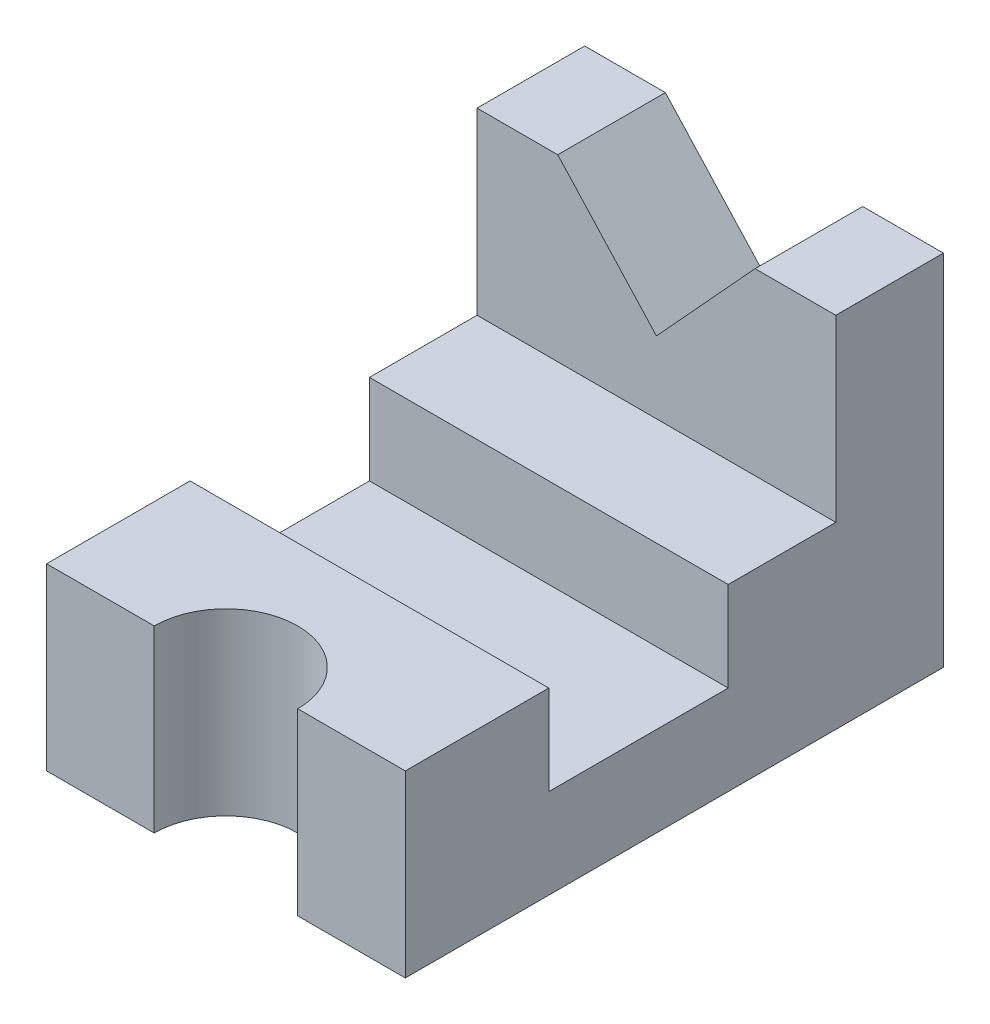
ISO-10303-21;
HEADER;
FILE_DESCRIPTION(('STEP AP214'),'2;1');
FILE_NAME('part.step','',(''),(''),'','','');
FILE_SCHEMA(('AUTOMOTIVE_DESIGN { 1 0 10303 214 1 1 1 1 }'));
ENDSEC;
DATA;
#1=APPLICATION_CONTEXT('core data for automotive mechanical design processes');
#2=APPLICATION_PROTOCOL_DEFINITION('international standard','automotive_design',2000,#1);
#3=PRODUCT_CONTEXT('',#1,'mechanical');
#4=PRODUCT('Part','Part','',(#3));
#5=PRODUCT_RELATED_PRODUCT_CATEGORY('part','',(#4));
#6=PRODUCT_DEFINITION_FORMATION('','',#4);
#7=PRODUCT_DEFINITION_CONTEXT('part definition',#1,'design');
#8=PRODUCT_DEFINITION('design','',#6,#7);
#9=PRODUCT_DEFINITION_SHAPE('','',#8);
#10=(LENGTH_UNIT() NAMED_UNIT(*) SI_UNIT(.MILLI.,.METRE.));
#11=(NAMED_UNIT(*) PLANE_ANGLE_UNIT() SI_UNIT($,.RADIAN.));
#12=(NAMED_UNIT(*) SI_UNIT($,.STERADIAN.) SOLID_ANGLE_UNIT());
#13=UNCERTAINTY_MEASURE_WITH_UNIT(LENGTH_MEASURE(1.E-05),#10,'distance_accuracy_value','');
#14=(GEOMETRIC_REPRESENTATION_CONTEXT(3) GLOBAL_UNCERTAINTY_ASSIGNED_CONTEXT((#13)) GLOBAL_UNIT_ASSIGNED_CONTEXT((#10,
#11,#12)) REPRESENTATION_CONTEXT('',''));
#15=CARTESIAN_POINT('',(0.,0.,0.));
#16=DIRECTION('',(0.,0.,1.));
#17=DIRECTION('',(1.,0.,0.));
#18=AXIS2_PLACEMENT_3D('',#15,#16,#17);
#19=CARTESIAN_POINT('',(60.,40.,12.));
#20=DIRECTION('',(0.,1.,0.));
#21=DIRECTION('',(0.,0.,1.));
#22=AXIS2_PLACEMENT_3D('',#19,#20,#21);
#23=PLANE('',#22);
#24=DIRECTION('',(0.,0.,1.));
#25=VECTOR('',#24,1.);
#26=CARTESIAN_POINT('',(51.,40.,-48.));
#27=LINE('',#26,#25);
#28=CARTESIAN_POINT('',(51.,40.,0.));
#29=VERTEX_POINT('',#28);
#30=CARTESIAN_POINT('',(51.,40.,12.));
#31=VERTEX_POINT('',#30);
#32=EDGE_CURVE('E157',#29,#31,#27,.T.);
#33=ORIENTED_EDGE('',*,*,#32,.T.);
#34=DIRECTION('',(1.,0.,0.));
#35=VECTOR('',#34,1.);
#36=CARTESIAN_POINT('',(60.,40.,12.));
#37=LINE('',#36,#35);
#38=CARTESIAN_POINT('',(60.,40.,12.));
#39=VERTEX_POINT('',#38);
#40=EDGE_CURVE('E168',#31,#39,#37,.T.);
#41=ORIENTED_EDGE('',*,*,#40,.T.);
#42=DIRECTION('',(0.,0.,-1.));
#43=VECTOR('',#42,1.);
#44=CARTESIAN_POINT('',(60.,40.,12.));
#45=LINE('',#44,#43);
#46=CARTESIAN_POINT('',(60.,40.,0.));
#47=VERTEX_POINT('',#46);
#48=EDGE_CURVE('E229',#39,#47,#45,.T.);
#49=ORIENTED_EDGE('',*,*,#48,.T.);
#50=DIRECTION('',(1.,0.,0.));
#51=VECTOR('',#50,1.);
#52=CARTESIAN_POINT('',(60.,40.,0.));
#53=LINE('',#52,#51);
#54=EDGE_CURVE('E221',#29,#47,#53,.T.);
#55=ORIENTED_EDGE('',*,*,#54,.F.);
#56=EDGE_LOOP('',(#33,#41,#49,#55));
#57=FACE_BOUND('',#56,.T.);
#58=ADVANCED_FACE('F44',(#57),#23,.T.);
#59=CARTESIAN_POINT('',(0.,20.,60.));
#60=DIRECTION('',(0.,-1.,0.));
#61=DIRECTION('',(0.,0.,-1.));
#62=AXIS2_PLACEMENT_3D('',#59,#60,#61);
#63=PLANE('',#62);
#64=DIRECTION('',(0.,0.,-1.));
#65=VECTOR('',#64,1.);
#66=CARTESIAN_POINT('',(60.,20.,60.));
#67=LINE('',#66,#65);
#68=CARTESIAN_POINT('',(60.,20.,60.));
#69=VERTEX_POINT('',#68);
#70=CARTESIAN_POINT('',(60.,20.,44.));
#71=VERTEX_POINT('',#70);
#72=EDGE_CURVE('E247',#69,#71,#67,.T.);
#73=ORIENTED_EDGE('',*,*,#72,.T.);
#74=DIRECTION('',(1.,0.,0.));
#75=VECTOR('',#74,1.);
#76=CARTESIAN_POINT('',(0.,20.,44.));
#77=LINE('',#76,#75);
#78=CARTESIAN_POINT('',(20.,20.,44.));
#79=VERTEX_POINT('',#78);
#80=EDGE_CURVE('E188',#79,#71,#77,.T.);
#81=ORIENTED_EDGE('',*,*,#80,.F.);
#82=DIRECTION('',(0.,0.,-1.));
#83=VECTOR('',#82,1.);
#84=CARTESIAN_POINT('',(20.,20.,60.));
#85=LINE('',#84,#83);
#86=CARTESIAN_POINT('',(20.,20.,60.));
#87=VERTEX_POINT('',#86);
#88=EDGE_CURVE('E206',#87,#79,#85,.T.);
#89=ORIENTED_EDGE('',*,*,#88,.F.);
#90=DIRECTION('',(-1.,0.,0.));
#91=VECTOR('',#90,1.);
#92=CARTESIAN_POINT('',(16.,20.,60.));
#93=LINE('',#92,#91);
#94=CARTESIAN_POINT('',(32.,20.,60.));
#95=VERTEX_POINT('',#94);
#96=EDGE_CURVE('E236',#95,#87,#93,.T.);
#97=ORIENTED_EDGE('',*,*,#96,.F.);
#98=CARTESIAN_POINT('',(40.,20.,60.));
#99=DIRECTION('',(0.,1.,0.));
#100=DIRECTION('',(0.,0.,1.));
#101=AXIS2_PLACEMENT_3D('',#98,#99,#100);
#102=CIRCLE('',#101,8.);
#103=CARTESIAN_POINT('',(48.,20.,60.));
#104=VERTEX_POINT('',#103);
#105=EDGE_CURVE('E186',#104,#95,#102,.T.);
#106=ORIENTED_EDGE('',*,*,#105,.F.);
#107=EDGE_CURVE('E239',#69,#104,#93,.T.);
#108=ORIENTED_EDGE('',*,*,#107,.F.);
#109=EDGE_LOOP('',(#73,#81,#89,#97,#106,#108));
#110=FACE_BOUND('',#109,.T.);
#111=ADVANCED_FACE('F280',(#110),#63,.F.);
#112=CARTESIAN_POINT('',(0.,0.,60.));
#113=DIRECTION('',(0.,0.,-1.));
#114=DIRECTION('',(-1.,0.,0.));
#115=AXIS2_PLACEMENT_3D('',#112,#113,#114);
#116=PLANE('',#115);
#117=DIRECTION('',(1.,0.,0.));
#118=VECTOR('',#117,1.);
#119=CARTESIAN_POINT('',(0.,0.,60.));
#120=LINE('',#119,#118);
#121=CARTESIAN_POINT('',(20.,0.,60.));
#122=VERTEX_POINT('',#121);
#123=CARTESIAN_POINT('',(32.,0.,60.));
#124=VERTEX_POINT('',#123);
#125=EDGE_CURVE('E232',#122,#124,#120,.T.);
#126=ORIENTED_EDGE('',*,*,#125,.T.);
#127=DIRECTION('',(0.,1.,0.));
#128=VECTOR('',#127,1.);
#129=CARTESIAN_POINT('',(32.,-40.,60.));
#130=LINE('',#129,#128);
#131=EDGE_CURVE('E258',#124,#95,#130,.T.);
#132=ORIENTED_EDGE('',*,*,#131,.T.);
#133=ORIENTED_EDGE('',*,*,#96,.T.);
#134=DIRECTION('',(0.,-1.,0.));
#135=VECTOR('',#134,1.);
#136=CARTESIAN_POINT('',(20.,20.,60.));
#137=LINE('',#136,#135);
#138=EDGE_CURVE('E196',#87,#122,#137,.T.);
#139=ORIENTED_EDGE('',*,*,#138,.T.);
#140=EDGE_LOOP('',(#126,#132,#133,#139));
#141=FACE_BOUND('',#140,.T.);
#142=ADVANCED_FACE('F313',(#141),#116,.F.);
#143=CARTESIAN_POINT('',(0.,0.,60.));
#144=DIRECTION('',(0.,1.,0.));
#145=DIRECTION('',(0.,0.,1.));
#146=AXIS2_PLACEMENT_3D('',#143,#144,#145);
#147=PLANE('',#146);
#148=CARTESIAN_POINT('',(48.,0.,60.));
#149=VERTEX_POINT('',#148);
#150=CARTESIAN_POINT('',(60.,0.,60.));
#151=VERTEX_POINT('',#150);
#152=EDGE_CURVE('E237',#149,#151,#120,.T.);
#153=ORIENTED_EDGE('',*,*,#152,.F.);
#154=CARTESIAN_POINT('',(40.,0.,60.));
#155=DIRECTION('',(0.,1.,0.));
#156=DIRECTION('',(0.,0.,1.));
#157=AXIS2_PLACEMENT_3D('',#154,#155,#156);
#158=CIRCLE('',#157,8.);
#159=EDGE_CURVE('E195',#149,#124,#158,.T.);
#160=ORIENTED_EDGE('',*,*,#159,.T.);
#161=ORIENTED_EDGE('',*,*,#125,.F.);
#162=DIRECTION('',(0.,0.,-1.));
#163=VECTOR('',#162,1.);
#164=CARTESIAN_POINT('',(20.,0.,60.));
#165=LINE('',#164,#163);
#166=CARTESIAN_POINT('',(20.,0.,0.));
#167=VERTEX_POINT('',#166);
#168=EDGE_CURVE('E205',#122,#167,#165,.T.);
#169=ORIENTED_EDGE('',*,*,#168,.T.);
#170=DIRECTION('',(1.,0.,0.));
#171=VECTOR('',#170,1.);
#172=CARTESIAN_POINT('',(0.,0.,0.));
#173=LINE('',#172,#171);
#174=CARTESIAN_POINT('',(60.,0.,0.));
#175=VERTEX_POINT('',#174);
#176=EDGE_CURVE('E228',#167,#175,#173,.T.);
#177=ORIENTED_EDGE('',*,*,#176,.T.);
#178=DIRECTION('',(0.,0.,-1.));
#179=VECTOR('',#178,1.);
#180=CARTESIAN_POINT('',(60.,0.,60.));
#181=LINE('',#180,#179);
#182=EDGE_CURVE('E250',#151,#175,#181,.T.);
#183=ORIENTED_EDGE('',*,*,#182,.F.);
#184=EDGE_LOOP('',(#153,#160,#161,#169,#177,#183));
#185=FACE_BOUND('',#184,.T.);
#186=ADVANCED_FACE('F50',(#185),#147,.F.);
#187=CARTESIAN_POINT('',(60.,20.,60.));
#188=DIRECTION('',(-1.,0.,0.));
#189=DIRECTION('',(0.,0.,1.));
#190=AXIS2_PLACEMENT_3D('',#187,#188,#189);
#191=PLANE('',#190);
#192=DIRECTION('',(0.,0.,-1.));
#193=VECTOR('',#192,1.);
#194=CARTESIAN_POINT('',(60.,10.,44.));
#195=LINE('',#194,#193);
#196=CARTESIAN_POINT('',(60.,10.,44.));
#197=VERTEX_POINT('',#196);
#198=CARTESIAN_POINT('',(60.,10.,24.));
#199=VERTEX_POINT('',#198);
#200=EDGE_CURVE('E179',#197,#199,#195,.T.);
#201=ORIENTED_EDGE('',*,*,#200,.F.);
#202=DIRECTION('',(0.,-1.,0.));
#203=VECTOR('',#202,1.);
#204=CARTESIAN_POINT('',(60.,20.,44.));
#205=LINE('',#204,#203);
#206=EDGE_CURVE('E181',#71,#197,#205,.T.);
#207=ORIENTED_EDGE('',*,*,#206,.F.);
#208=ORIENTED_EDGE('',*,*,#72,.F.);
#209=DIRECTION('',(0.,1.,0.));
#210=VECTOR('',#209,1.);
#211=CARTESIAN_POINT('',(60.,20.,60.));
#212=LINE('',#211,#210);
#213=EDGE_CURVE('E235',#151,#69,#212,.T.);
#214=ORIENTED_EDGE('',*,*,#213,.F.);
#215=ORIENTED_EDGE('',*,*,#182,.T.);
#216=DIRECTION('',(0.,1.,0.));
#217=VECTOR('',#216,1.);
#218=CARTESIAN_POINT('',(60.,20.,0.));
#219=LINE('',#218,#217);
#220=EDGE_CURVE('E241',#175,#47,#219,.T.);
#221=ORIENTED_EDGE('',*,*,#220,.T.);
#222=ORIENTED_EDGE('',*,*,#48,.F.);
#223=DIRECTION('',(0.,-1.,0.));
#224=VECTOR('',#223,1.);
#225=CARTESIAN_POINT('',(60.,20.,12.));
#226=LINE('',#225,#224);
#227=CARTESIAN_POINT('',(60.,20.,12.));
#228=VERTEX_POINT('',#227);
#229=EDGE_CURVE('E217',#39,#228,#226,.T.);
#230=ORIENTED_EDGE('',*,*,#229,.T.);
#231=CARTESIAN_POINT('',(60.,20.,24.));
#232=VERTEX_POINT('',#231);
#233=EDGE_CURVE('E244',#232,#228,#67,.T.);
#234=ORIENTED_EDGE('',*,*,#233,.F.);
#235=DIRECTION('',(0.,1.,0.));
#236=VECTOR('',#235,1.);
#237=CARTESIAN_POINT('',(60.,10.,24.));
#238=LINE('',#237,#236);
#239=EDGE_CURVE('E182',#199,#232,#238,.T.);
#240=ORIENTED_EDGE('',*,*,#239,.F.);
#241=EDGE_LOOP('',(#201,#207,#208,#214,#215,#221,#222,#230,#234,#240));
#242=FACE_BOUND('',#241,.T.);
#243=ADVANCED_FACE('F284',(#242),#191,.F.);
#244=CARTESIAN_POINT('',(20.,20.,24.));
#245=VERTEX_POINT('',#244);
#246=CARTESIAN_POINT('',(20.,20.,12.));
#247=VERTEX_POINT('',#246);
#248=EDGE_CURVE('E203',#245,#247,#85,.T.);
#249=ORIENTED_EDGE('',*,*,#248,.F.);
#250=DIRECTION('',(1.,0.,0.));
#251=VECTOR('',#250,1.);
#252=CARTESIAN_POINT('',(0.,20.,24.));
#253=LINE('',#252,#251);
#254=EDGE_CURVE('E69',#245,#232,#253,.T.);
#255=ORIENTED_EDGE('',*,*,#254,.T.);
#256=ORIENTED_EDGE('',*,*,#233,.T.);
#257=DIRECTION('',(-1.,0.,0.));
#258=VECTOR('',#257,1.);
#259=CARTESIAN_POINT('',(20.,20.,12.));
#260=LINE('',#259,#258);
#261=EDGE_CURVE('E207',#228,#247,#260,.T.);
#262=ORIENTED_EDGE('',*,*,#261,.T.);
#263=EDGE_LOOP('',(#249,#255,#256,#262));
#264=FACE_BOUND('',#263,.T.);
#265=ADVANCED_FACE('F288',(#264),#63,.F.);
#266=ORIENTED_EDGE('',*,*,#107,.T.);
#267=DIRECTION('',(0.,1.,0.));
#268=VECTOR('',#267,1.);
#269=CARTESIAN_POINT('',(48.,-40.,60.));
#270=LINE('',#269,#268);
#271=EDGE_CURVE('E251',#104,#149,#270,.F.);
#272=ORIENTED_EDGE('',*,*,#271,.T.);
#273=ORIENTED_EDGE('',*,*,#152,.T.);
#274=ORIENTED_EDGE('',*,*,#213,.T.);
#275=EDGE_LOOP('',(#266,#272,#273,#274));
#276=FACE_BOUND('',#275,.T.);
#277=ADVANCED_FACE('F321',(#276),#116,.F.);
#278=CARTESIAN_POINT('',(0.,0.,0.));
#279=DIRECTION('',(0.,0.,-1.));
#280=DIRECTION('',(-1.,0.,0.));
#281=AXIS2_PLACEMENT_3D('',#278,#279,#280);
#282=PLANE('',#281);
#283=DIRECTION('',(-0.675724628517346,-0.737154140200742,0.));
#284=VECTOR('',#283,1.);
#285=CARTESIAN_POINT('',(7.78867924528303,-7.13962264150944,0.));
#286=LINE('',#285,#284);
#287=CARTESIAN_POINT('',(40.,28.,0.));
#288=VERTEX_POINT('',#287);
#289=EDGE_CURVE('E160',#29,#288,#286,.T.);
#290=ORIENTED_EDGE('',*,*,#289,.F.);
#291=ORIENTED_EDGE('',*,*,#54,.T.);
#292=ORIENTED_EDGE('',*,*,#220,.F.);
#293=ORIENTED_EDGE('',*,*,#176,.F.);
#294=DIRECTION('',(0.,1.,0.));
#295=VECTOR('',#294,1.);
#296=CARTESIAN_POINT('',(20.,40.,0.));
#297=LINE('',#296,#295);
#298=CARTESIAN_POINT('',(20.,40.,0.));
#299=VERTEX_POINT('',#298);
#300=EDGE_CURVE('E202',#167,#299,#297,.T.);
#301=ORIENTED_EDGE('',*,*,#300,.T.);
#302=CARTESIAN_POINT('',(29.,40.,0.));
#303=VERTEX_POINT('',#302);
#304=EDGE_CURVE('E213',#299,#303,#53,.T.);
#305=ORIENTED_EDGE('',*,*,#304,.T.);
#306=DIRECTION('',(-0.675724628517346,0.737154140200742,0.));
#307=VECTOR('',#306,1.);
#308=CARTESIAN_POINT('',(35.6830188679245,32.7094339622641,0.));
#309=LINE('',#308,#307);
#310=EDGE_CURVE('E171',#288,#303,#309,.T.);
#311=ORIENTED_EDGE('',*,*,#310,.F.);
#312=EDGE_LOOP('',(#290,#291,#292,#293,#301,#305,#311));
#313=FACE_BOUND('',#312,.T.);
#314=ADVANCED_FACE('F302',(#313),#282,.T.);
#315=DIRECTION('',(0.,0.,1.));
#316=VECTOR('',#315,1.);
#317=CARTESIAN_POINT('',(29.,40.,-48.));
#318=LINE('',#317,#316);
#319=CARTESIAN_POINT('',(29.,40.,12.));
#320=VERTEX_POINT('',#319);
#321=EDGE_CURVE('E58',#303,#320,#318,.T.);
#322=ORIENTED_EDGE('',*,*,#321,.F.);
#323=ORIENTED_EDGE('',*,*,#304,.F.);
#324=DIRECTION('',(0.,0.,-1.));
#325=VECTOR('',#324,1.);
#326=CARTESIAN_POINT('',(20.,40.,12.));
#327=LINE('',#326,#325);
#328=CARTESIAN_POINT('',(20.,40.,12.));
#329=VERTEX_POINT('',#328);
#330=EDGE_CURVE('E222',#329,#299,#327,.T.);
#331=ORIENTED_EDGE('',*,*,#330,.F.);
#332=EDGE_CURVE('E216',#329,#320,#37,.T.);
#333=ORIENTED_EDGE('',*,*,#332,.T.);
#334=EDGE_LOOP('',(#322,#323,#331,#333));
#335=FACE_BOUND('',#334,.T.);
#336=ADVANCED_FACE('F291',(#335),#23,.T.);
#337=CARTESIAN_POINT('',(20.,40.,12.));
#338=DIRECTION('',(-1.,0.,0.));
#339=DIRECTION('',(0.,0.,1.));
#340=AXIS2_PLACEMENT_3D('',#337,#338,#339);
#341=PLANE('',#340);
#342=DIRECTION('',(0.,1.,0.));
#343=VECTOR('',#342,1.);
#344=CARTESIAN_POINT('',(20.,40.,44.));
#345=LINE('',#344,#343);
#346=CARTESIAN_POINT('',(20.,10.,44.));
#347=VERTEX_POINT('',#346);
#348=EDGE_CURVE('E11',#347,#79,#345,.T.);
#349=ORIENTED_EDGE('',*,*,#348,.F.);
#350=DIRECTION('',(0.,0.,1.));
#351=VECTOR('',#350,1.);
#352=CARTESIAN_POINT('',(20.,10.,12.));
#353=LINE('',#352,#351);
#354=CARTESIAN_POINT('',(20.,10.,24.));
#355=VERTEX_POINT('',#354);
#356=EDGE_CURVE('E52',#355,#347,#353,.T.);
#357=ORIENTED_EDGE('',*,*,#356,.F.);
#358=DIRECTION('',(0.,-1.,0.));
#359=VECTOR('',#358,1.);
#360=CARTESIAN_POINT('',(20.,40.,24.));
#361=LINE('',#360,#359);
#362=EDGE_CURVE('E259',#245,#355,#361,.T.);
#363=ORIENTED_EDGE('',*,*,#362,.F.);
#364=ORIENTED_EDGE('',*,*,#248,.T.);
#365=DIRECTION('',(0.,1.,0.));
#366=VECTOR('',#365,1.);
#367=CARTESIAN_POINT('',(20.,40.,12.));
#368=LINE('',#367,#366);
#369=EDGE_CURVE('E215',#247,#329,#368,.T.);
#370=ORIENTED_EDGE('',*,*,#369,.T.);
#371=ORIENTED_EDGE('',*,*,#330,.T.);
#372=ORIENTED_EDGE('',*,*,#300,.F.);
#373=ORIENTED_EDGE('',*,*,#168,.F.);
#374=ORIENTED_EDGE('',*,*,#138,.F.);
#375=ORIENTED_EDGE('',*,*,#88,.T.);
#376=EDGE_LOOP('',(#349,#357,#363,#364,#370,#371,#372,#373,#374,#375));
#377=FACE_BOUND('',#376,.T.);
#378=ADVANCED_FACE('F275',(#377),#341,.T.);
#379=CARTESIAN_POINT('',(0.,0.,12.));
#380=DIRECTION('',(0.,0.,1.));
#381=DIRECTION('',(1.,0.,0.));
#382=AXIS2_PLACEMENT_3D('',#379,#380,#381);
#383=PLANE('',#382);
#384=DIRECTION('',(0.675724628517346,0.737154140200742,0.));
#385=VECTOR('',#384,1.);
#386=CARTESIAN_POINT('',(51.,40.,12.));
#387=LINE('',#386,#385);
#388=CARTESIAN_POINT('',(40.,28.,12.));
#389=VERTEX_POINT('',#388);
#390=EDGE_CURVE('E152',#389,#31,#387,.T.);
#391=ORIENTED_EDGE('',*,*,#390,.F.);
#392=DIRECTION('',(0.675724628517346,-0.737154140200741,0.));
#393=VECTOR('',#392,1.);
#394=CARTESIAN_POINT('',(29.,40.,12.));
#395=LINE('',#394,#393);
#396=EDGE_CURVE('E161',#320,#389,#395,.T.);
#397=ORIENTED_EDGE('',*,*,#396,.F.);
#398=ORIENTED_EDGE('',*,*,#332,.F.);
#399=ORIENTED_EDGE('',*,*,#369,.F.);
#400=ORIENTED_EDGE('',*,*,#261,.F.);
#401=ORIENTED_EDGE('',*,*,#229,.F.);
#402=ORIENTED_EDGE('',*,*,#40,.F.);
#403=EDGE_LOOP('',(#391,#397,#398,#399,#400,#401,#402));
#404=FACE_BOUND('',#403,.T.);
#405=ADVANCED_FACE('F169',(#404),#383,.T.);
#406=CARTESIAN_POINT('',(40.,-40.,60.));
#407=DIRECTION('',(0.,1.,0.));
#408=DIRECTION('',(0.,0.,1.));
#409=AXIS2_PLACEMENT_3D('',#406,#407,#408);
#410=CYLINDRICAL_SURFACE('',#409,8.);
#411=ORIENTED_EDGE('',*,*,#271,.F.);
#412=ORIENTED_EDGE('',*,*,#105,.T.);
#413=ORIENTED_EDGE('',*,*,#131,.F.);
#414=ORIENTED_EDGE('',*,*,#159,.F.);
#415=EDGE_LOOP('',(#411,#412,#413,#414));
#416=FACE_BOUND('',#415,.T.);
#417=ADVANCED_FACE('F344',(#416),#410,.F.);
#418=CARTESIAN_POINT('',(0.,10.,44.));
#419=DIRECTION('',(0.,-1.,0.));
#420=DIRECTION('',(0.,0.,-1.));
#421=AXIS2_PLACEMENT_3D('',#418,#419,#420);
#422=PLANE('',#421);
#423=ORIENTED_EDGE('',*,*,#356,.T.);
#424=DIRECTION('',(1.,0.,0.));
#425=VECTOR('',#424,1.);
#426=CARTESIAN_POINT('',(0.,10.,44.));
#427=LINE('',#426,#425);
#428=EDGE_CURVE('E189',#347,#197,#427,.T.);
#429=ORIENTED_EDGE('',*,*,#428,.T.);
#430=ORIENTED_EDGE('',*,*,#200,.T.);
#431=DIRECTION('',(1.,0.,0.));
#432=VECTOR('',#431,1.);
#433=CARTESIAN_POINT('',(0.,10.,24.));
#434=LINE('',#433,#432);
#435=EDGE_CURVE('E187',#355,#199,#434,.T.);
#436=ORIENTED_EDGE('',*,*,#435,.F.);
#437=EDGE_LOOP('',(#423,#429,#430,#436));
#438=FACE_BOUND('',#437,.T.);
#439=ADVANCED_FACE('F262',(#438),#422,.F.);
#440=CARTESIAN_POINT('',(0.,20.,44.));
#441=DIRECTION('',(0.,0.,1.));
#442=DIRECTION('',(1.,0.,0.));
#443=AXIS2_PLACEMENT_3D('',#440,#441,#442);
#444=PLANE('',#443);
#445=ORIENTED_EDGE('',*,*,#348,.T.);
#446=ORIENTED_EDGE('',*,*,#80,.T.);
#447=ORIENTED_EDGE('',*,*,#206,.T.);
#448=ORIENTED_EDGE('',*,*,#428,.F.);
#449=EDGE_LOOP('',(#445,#446,#447,#448));
#450=FACE_BOUND('',#449,.T.);
#451=ADVANCED_FACE('F268',(#450),#444,.F.);
#452=CARTESIAN_POINT('',(0.,10.,24.));
#453=DIRECTION('',(0.,0.,-1.));
#454=DIRECTION('',(-1.,0.,0.));
#455=AXIS2_PLACEMENT_3D('',#452,#453,#454);
#456=PLANE('',#455);
#457=ORIENTED_EDGE('',*,*,#362,.T.);
#458=ORIENTED_EDGE('',*,*,#435,.T.);
#459=ORIENTED_EDGE('',*,*,#239,.T.);
#460=ORIENTED_EDGE('',*,*,#254,.F.);
#461=EDGE_LOOP('',(#457,#458,#459,#460));
#462=FACE_BOUND('',#461,.T.);
#463=ADVANCED_FACE('F286',(#462),#456,.F.);
#464=CARTESIAN_POINT('',(51.,40.,-48.));
#465=DIRECTION('',(0.737154140200742,-0.675724628517346,0.));
#466=DIRECTION('',(0.675724628517346,0.737154140200742,0.));
#467=AXIS2_PLACEMENT_3D('',#464,#465,#466);
#468=PLANE('',#467);
#469=ORIENTED_EDGE('',*,*,#289,.T.);
#470=DIRECTION('',(0.,0.,1.));
#471=VECTOR('',#470,1.);
#472=CARTESIAN_POINT('',(40.,28.,-48.));
#473=LINE('',#472,#471);
#474=EDGE_CURVE('E151',#288,#389,#473,.T.);
#475=ORIENTED_EDGE('',*,*,#474,.T.);
#476=ORIENTED_EDGE('',*,*,#390,.T.);
#477=ORIENTED_EDGE('',*,*,#32,.F.);
#478=EDGE_LOOP('',(#469,#475,#476,#477));
#479=FACE_BOUND('',#478,.T.);
#480=ADVANCED_FACE('F155',(#479),#468,.F.);
#481=CARTESIAN_POINT('',(29.,40.,-48.));
#482=DIRECTION('',(-0.737154140200741,-0.675724628517346,0.));
#483=DIRECTION('',(0.675724628517346,-0.737154140200742,0.));
#484=AXIS2_PLACEMENT_3D('',#481,#482,#483);
#485=PLANE('',#484);
#486=ORIENTED_EDGE('',*,*,#310,.T.);
#487=ORIENTED_EDGE('',*,*,#321,.T.);
#488=ORIENTED_EDGE('',*,*,#396,.T.);
#489=ORIENTED_EDGE('',*,*,#474,.F.);
#490=EDGE_LOOP('',(#486,#487,#488,#489));
#491=FACE_BOUND('',#490,.T.);
#492=ADVANCED_FACE('F165',(#491),#485,.F.);
#493=CLOSED_SHELL('',(#58,#111,#142,#186,#243,#265,#277,#314,#336,#378,#405,#417,#439,#451,#463,
#480,#492));
#494=MANIFOLD_SOLID_BREP('B2',#493);
#495=ADVANCED_BREP_SHAPE_REPRESENTATION('',(#18,#494),#14);
#496=SHAPE_DEFINITION_REPRESENTATION(#9,#495);
ENDSEC;
END-ISO-10303-21;
